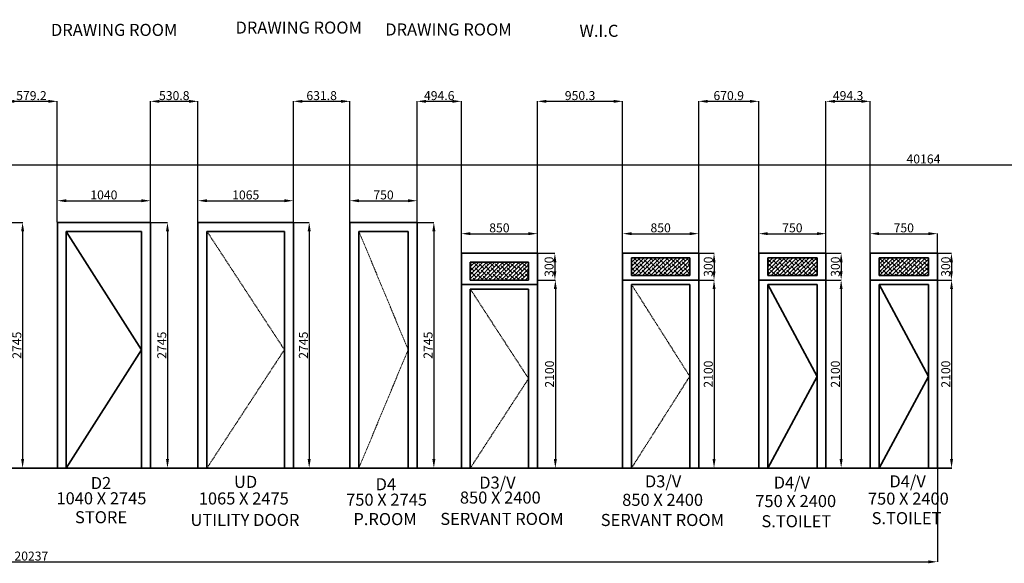
# Model space of a CAD drawing. Units: millimetres. Extents: x -850 to 42148, y -7352 to 4589.
# Tile 2 of 4: x 11314 to 22310, y -7352 to -1278. Entities that reach past the tile are written whole.
import ezdxf

# ---------------------------------------------------------------- set-up
doc = ezdxf.new("R2010")
doc.units = ezdxf.units.MM
doc.linetypes.add('DASHED', pattern=[19.05, 12.7, -6.35])
for name, color, linetype, lineweight in [('A-ANNO-DIMS', 2, 'Continuous', 18), ('A-ANNO-TEXT', 7, 'Continuous', 18), ('A-DOOR', 3, 'Continuous', 35), ('A-DOOR-OPNG', 3, 'DASHED', 18), ('A-DOOR-PATT', 252, 'Continuous', 13)]:
    doc.layers.add(name, color=color, linetype=linetype, lineweight=lineweight)
doc.styles.get("Standard").update_dxf_attribs({"font": 'arial.ttf'})
doc.dimstyles.new('ISO-25', dxfattribs={"dimtxt": 100, "dimasz": 100, "dimexe": 1.25, "dimexo": 0.625, "dimtad": 1, "dimtxsty": 'Standard', "dimcen": 2.5, "dimadec": 0, "dimazin": 0, "dimtfac": 1, "dimtmove": 0, "dimatfit": 3, "dimfxl": 1, "dimarcsym": 0})

# ---------------------------------------------------------------- blocks, each defined once
blk = doc.blocks.new('*D38')
at = {"layer": 'A-ANNO-DIMS', "color": 0, "lineweight": -2, "transparency": 16777216}
for p, q in [((11156, -3543), (11347, -3543)), ((11346, -3643), (11346, -6188)), ((11156, -6288), (11347, -6288))]:
    blk.add_line(p, q, dxfattribs=at)
at = {"layer": 'A-ANNO-DIMS', "color": 0, "lineweight": 30, "transparency": 16777216}
for points in [[(11330, -3643), (11363, -3643), (11346, -3543)], [(11330, -6188), (11363, -6188), (11346, -6288)]]:
    blk.add_solid(points, dxfattribs=at)
at = {"layer": 'Defpoints', "color": 0, "lineweight": 30, "transparency": 16777216}
for p in [(11155, -3543), (11155, -6288), (11346, -6288)]:
    blk.add_point(p, dxfattribs=at)
at = {"layer": 'A-ANNO-DIMS', "color": 0, "transparency": 16777216, "insert": (11295, -4915), "char_height": 100, "attachment_point": 5, "rotation": 90}
blk.add_mtext('2745', dxfattribs=at)
blk = doc.blocks.new('*D39')
at = {"layer": 'A-ANNO-DIMS', "color": 0, "lineweight": -2, "transparency": 16777216}
for p, q in [((11734, -3542), (11734, -3299)), ((11834, -3301), (12674, -3301)), ((12774, -3542), (12774, -3299))]:
    blk.add_line(p, q, dxfattribs=at)
at = {"layer": 'A-ANNO-DIMS', "color": 0, "lineweight": 30, "transparency": 16777216}
for points in [[(11834, -3284), (11834, -3317), (11734, -3301)], [(12674, -3284), (12674, -3317), (12774, -3301)]]:
    blk.add_solid(points, dxfattribs=at)
at = {"layer": 'Defpoints', "color": 0, "lineweight": 30, "transparency": 16777216}
for p in [(12774, -3301), (11734, -3543), (12774, -3543)]:
    blk.add_point(p, dxfattribs=at)
at = {"layer": 'A-ANNO-DIMS', "color": 0, "transparency": 16777216, "insert": (12254, -3249), "char_height": 100, "attachment_point": 5}
blk.add_mtext('1040', dxfattribs=at)
blk = doc.blocks.new('*D40')
at = {"layer": 'A-ANNO-DIMS', "color": 0, "lineweight": -2, "transparency": 16777216}
for p, q in [((12775, -3543), (12966, -3543)), ((12964, -3643), (12964, -6188)), ((12775, -6288), (12966, -6288))]:
    blk.add_line(p, q, dxfattribs=at)
at = {"layer": 'A-ANNO-DIMS', "color": 0, "lineweight": 30, "transparency": 16777216}
for points in [[(12948, -3643), (12981, -3643), (12964, -3543)], [(12948, -6188), (12981, -6188), (12964, -6288)]]:
    blk.add_solid(points, dxfattribs=at)
at = {"layer": 'Defpoints', "color": 0, "lineweight": 30, "transparency": 16777216}
for p in [(12774, -3543), (12774, -6288), (12964, -6288)]:
    blk.add_point(p, dxfattribs=at)
at = {"layer": 'A-ANNO-DIMS', "color": 0, "transparency": 16777216, "insert": (12913, -4915), "char_height": 100, "attachment_point": 5, "rotation": 90}
blk.add_mtext('2745', dxfattribs=at)
blk = doc.blocks.new('*D41')
at = {"layer": 'A-ANNO-DIMS', "color": 0, "lineweight": -2, "transparency": 16777216}
for p, q in [((13305, -3542), (13305, -3299)), ((13405, -3301), (14270, -3301)), ((14370, -3542), (14370, -3299))]:
    blk.add_line(p, q, dxfattribs=at)
at = {"layer": 'A-ANNO-DIMS', "color": 0, "lineweight": 30, "transparency": 16777216}
for points in [[(13405, -3284), (13405, -3317), (13305, -3301)], [(14270, -3284), (14270, -3317), (14370, -3301)]]:
    blk.add_solid(points, dxfattribs=at)
at = {"layer": 'Defpoints', "color": 0, "lineweight": 30, "transparency": 16777216}
for p in [(14370, -3301), (13305, -3543), (14370, -3543)]:
    blk.add_point(p, dxfattribs=at)
at = {"layer": 'A-ANNO-DIMS', "color": 0, "transparency": 16777216, "insert": (13838, -3249), "char_height": 100, "attachment_point": 5}
blk.add_mtext('1065', dxfattribs=at)
blk = doc.blocks.new('*D42')
at = {"layer": 'A-ANNO-DIMS', "color": 0, "lineweight": -2, "transparency": 16777216}
for p, q in [((14371, -3543), (14548, -3543)), ((14547, -3643), (14547, -6188)), ((14371, -6288), (14548, -6288))]:
    blk.add_line(p, q, dxfattribs=at)
at = {"layer": 'A-ANNO-DIMS', "color": 0, "lineweight": 30, "transparency": 16777216}
for points in [[(14530, -3643), (14564, -3643), (14547, -3543)], [(14530, -6188), (14564, -6188), (14547, -6288)]]:
    blk.add_solid(points, dxfattribs=at)
at = {"layer": 'Defpoints', "color": 0, "lineweight": 30, "transparency": 16777216}
for p in [(14370, -3543), (14370, -6288), (14547, -6288)]:
    blk.add_point(p, dxfattribs=at)
at = {"layer": 'A-ANNO-DIMS', "color": 0, "transparency": 16777216, "insert": (14495, -4915), "char_height": 100, "attachment_point": 5, "rotation": 90}
blk.add_mtext('2745', dxfattribs=at)
blk = doc.blocks.new('*D43')
at = {"layer": 'A-ANNO-DIMS', "color": 0, "lineweight": -2, "transparency": 16777216}
for p, q in [((15002, -3542), (15002, -3299)), ((15102, -3301), (15652, -3301)), ((15752, -3542), (15752, -3299))]:
    blk.add_line(p, q, dxfattribs=at)
at = {"layer": 'A-ANNO-DIMS', "color": 0, "lineweight": 30, "transparency": 16777216}
for points in [[(15102, -3284), (15102, -3317), (15002, -3301)], [(15652, -3284), (15652, -3317), (15752, -3301)]]:
    blk.add_solid(points, dxfattribs=at)
at = {"layer": 'Defpoints', "color": 0, "lineweight": 30, "transparency": 16777216}
for p in [(15752, -3301), (15002, -3543), (15752, -3543)]:
    blk.add_point(p, dxfattribs=at)
at = {"layer": 'A-ANNO-DIMS', "color": 0, "transparency": 16777216, "insert": (15377, -3249), "char_height": 100, "attachment_point": 5}
blk.add_mtext('750', dxfattribs=at)
blk = doc.blocks.new('*D44')
at = {"layer": 'A-ANNO-DIMS', "color": 0, "lineweight": -2, "transparency": 16777216}
for p, q in [((15752, -3543), (15940, -3543)), ((15939, -3643), (15939, -6188)), ((15752, -6288), (15940, -6288))]:
    blk.add_line(p, q, dxfattribs=at)
at = {"layer": 'A-ANNO-DIMS', "color": 0, "lineweight": 30, "transparency": 16777216}
for points in [[(15922, -3643), (15956, -3643), (15939, -3543)], [(15922, -6188), (15956, -6188), (15939, -6288)]]:
    blk.add_solid(points, dxfattribs=at)
at = {"layer": 'Defpoints', "color": 0, "lineweight": 30, "transparency": 16777216}
for p in [(15752, -3543), (15752, -6288), (15939, -6288)]:
    blk.add_point(p, dxfattribs=at)
at = {"layer": 'A-ANNO-DIMS', "color": 0, "transparency": 16777216, "insert": (15887, -4915), "char_height": 100, "attachment_point": 5, "rotation": 90}
blk.add_mtext('2745', dxfattribs=at)
blk = doc.blocks.new('*D45')
at = {"layer": 'A-ANNO-DIMS', "color": 0, "lineweight": -2, "transparency": 16777216}
for p, q in [((16246, -3887), (16246, -3667)), ((16346, -3669), (16996, -3669)), ((17096, -3887), (17096, -3667))]:
    blk.add_line(p, q, dxfattribs=at)
at = {"layer": 'A-ANNO-DIMS', "color": 0, "lineweight": 30, "transparency": 16777216}
for points in [[(16346, -3652), (16346, -3685), (16246, -3669)], [(16996, -3652), (16996, -3685), (17096, -3669)]]:
    blk.add_solid(points, dxfattribs=at)
at = {"layer": 'Defpoints', "color": 0, "lineweight": 30, "transparency": 16777216}
for p in [(17096, -3669), (16246, -3888), (17096, -3888)]:
    blk.add_point(p, dxfattribs=at)
at = {"layer": 'A-ANNO-DIMS', "color": 0, "transparency": 16777216, "insert": (16671, -3617), "char_height": 100, "attachment_point": 5}
blk.add_mtext('850', dxfattribs=at)
blk = doc.blocks.new('*D46')
at = {"layer": 'A-ANNO-DIMS', "color": 0, "lineweight": -2, "transparency": 16777216}
for p, q in [((17097, -4188), (17297, -4188)), ((17296, -4288), (17296, -6188)), ((17097, -6288), (17297, -6288))]:
    blk.add_line(p, q, dxfattribs=at)
at = {"layer": 'A-ANNO-DIMS', "color": 0, "lineweight": 30, "transparency": 16777216}
for points in [[(17279, -4288), (17313, -4288), (17296, -4188)], [(17279, -6188), (17313, -6188), (17296, -6288)]]:
    blk.add_solid(points, dxfattribs=at)
at = {"layer": 'Defpoints', "color": 0, "lineweight": 30, "transparency": 16777216}
for p in [(17096, -4188), (17096, -6288), (17296, -6288)]:
    blk.add_point(p, dxfattribs=at)
at = {"layer": 'A-ANNO-DIMS', "color": 0, "transparency": 16777216, "insert": (17244, -5238), "char_height": 100, "attachment_point": 5, "rotation": 90}
blk.add_mtext('2100', dxfattribs=at)
blk = doc.blocks.new('*D47')
at = {"layer": 'A-ANNO-DIMS', "color": 0, "lineweight": -2, "transparency": 16777216}
for p, q in [((17097, -3888), (17292, -3888)), ((17291, -3988), (17291, -4088)), ((17097, -4188), (17292, -4188))]:
    blk.add_line(p, q, dxfattribs=at)
at = {"layer": 'A-ANNO-DIMS', "color": 0, "lineweight": 30, "transparency": 16777216}
for points in [[(17274, -3988), (17307, -3988), (17291, -3888)], [(17274, -4088), (17307, -4088), (17291, -4188)]]:
    blk.add_solid(points, dxfattribs=at)
at = {"layer": 'Defpoints', "color": 0, "lineweight": 30, "transparency": 16777216}
for p in [(17096, -3888), (17096, -4188), (17291, -4188)]:
    blk.add_point(p, dxfattribs=at)
at = {"layer": 'A-ANNO-DIMS', "color": 0, "transparency": 16777216, "insert": (17239, -4038), "char_height": 100, "attachment_point": 5, "rotation": 90}
blk.add_mtext('300', dxfattribs=at)
blk = doc.blocks.new('*D48')
at = {"layer": 'A-ANNO-DIMS', "color": 0, "lineweight": -2, "transparency": 16777216}
for p, q in [((18047, -3887), (18047, -3667)), ((18147, -3669), (18797, -3669)), ((18897, -3887), (18897, -3667))]:
    blk.add_line(p, q, dxfattribs=at)
at = {"layer": 'A-ANNO-DIMS', "color": 0, "lineweight": 30, "transparency": 16777216}
for points in [[(18147, -3652), (18147, -3685), (18047, -3669)], [(18797, -3652), (18797, -3685), (18897, -3669)]]:
    blk.add_solid(points, dxfattribs=at)
at = {"layer": 'Defpoints', "color": 0, "lineweight": 30, "transparency": 16777216}
for p in [(18897, -3669), (18047, -3888), (18897, -3888)]:
    blk.add_point(p, dxfattribs=at)
at = {"layer": 'A-ANNO-DIMS', "color": 0, "transparency": 16777216, "insert": (18472, -3617), "char_height": 100, "attachment_point": 5}
blk.add_mtext('850', dxfattribs=at)
blk = doc.blocks.new('*D49')
at = {"layer": 'A-ANNO-DIMS', "color": 0, "lineweight": -2, "transparency": 16777216}
for p, q in [((18897, -3888), (19070, -3888)), ((19068, -3988), (19068, -4088)), ((18897, -4188), (19070, -4188))]:
    blk.add_line(p, q, dxfattribs=at)
at = {"layer": 'A-ANNO-DIMS', "color": 0, "lineweight": 30, "transparency": 16777216}
for points in [[(19052, -3988), (19085, -3988), (19068, -3888)], [(19052, -4088), (19085, -4088), (19068, -4188)]]:
    blk.add_solid(points, dxfattribs=at)
at = {"layer": 'Defpoints', "color": 0, "lineweight": 30, "transparency": 16777216}
for p in [(18897, -3888), (18897, -4188), (19068, -4188)]:
    blk.add_point(p, dxfattribs=at)
at = {"layer": 'A-ANNO-DIMS', "color": 0, "transparency": 16777216, "insert": (19017, -4038), "char_height": 100, "attachment_point": 5, "rotation": 90}
blk.add_mtext('300', dxfattribs=at)
blk = doc.blocks.new('*D50')
at = {"layer": 'A-ANNO-DIMS', "color": 0, "lineweight": -2, "transparency": 16777216}
for p, q in [((18897, -4188), (19070, -4188)), ((19068, -4288), (19068, -6188)), ((18897, -6288), (19070, -6288))]:
    blk.add_line(p, q, dxfattribs=at)
at = {"layer": 'A-ANNO-DIMS', "color": 0, "lineweight": 30, "transparency": 16777216}
for points in [[(19052, -4288), (19085, -4288), (19068, -4188)], [(19052, -6188), (19085, -6188), (19068, -6288)]]:
    blk.add_solid(points, dxfattribs=at)
at = {"layer": 'Defpoints', "color": 0, "lineweight": 30, "transparency": 16777216}
for p in [(18897, -4188), (18897, -6288), (19068, -6288)]:
    blk.add_point(p, dxfattribs=at)
at = {"layer": 'A-ANNO-DIMS', "color": 0, "transparency": 16777216, "insert": (19017, -5238), "char_height": 100, "attachment_point": 5, "rotation": 90}
blk.add_mtext('2100', dxfattribs=at)
blk = doc.blocks.new('*D51')
at = {"layer": 'A-ANNO-DIMS', "color": 0, "lineweight": -2, "transparency": 16777216}
for p, q in [((19568, -3887), (19568, -3667)), ((19668, -3669), (20218, -3669)), ((20318, -3887), (20318, -3667))]:
    blk.add_line(p, q, dxfattribs=at)
at = {"layer": 'A-ANNO-DIMS', "color": 0, "lineweight": 30, "transparency": 16777216}
for points in [[(19668, -3652), (19668, -3685), (19568, -3669)], [(20218, -3652), (20218, -3685), (20318, -3669)]]:
    blk.add_solid(points, dxfattribs=at)
at = {"layer": 'Defpoints', "color": 0, "lineweight": 30, "transparency": 16777216}
for p in [(20318, -3669), (19568, -3888), (20318, -3888)]:
    blk.add_point(p, dxfattribs=at)
at = {"layer": 'A-ANNO-DIMS', "color": 0, "transparency": 16777216, "insert": (19943, -3617), "char_height": 100, "attachment_point": 5}
blk.add_mtext('750', dxfattribs=at)
blk = doc.blocks.new('*D52')
at = {"layer": 'A-ANNO-DIMS', "color": 0, "lineweight": -2, "transparency": 16777216}
for p, q in [((20318, -3888), (20489, -3888)), ((20488, -3988), (20488, -4088)), ((20318, -4188), (20489, -4188))]:
    blk.add_line(p, q, dxfattribs=at)
at = {"layer": 'A-ANNO-DIMS', "color": 0, "lineweight": 30, "transparency": 16777216}
for points in [[(20471, -3988), (20504, -3988), (20488, -3888)], [(20471, -4088), (20504, -4088), (20488, -4188)]]:
    blk.add_solid(points, dxfattribs=at)
at = {"layer": 'Defpoints', "color": 0, "lineweight": 30, "transparency": 16777216}
for p in [(20318, -3888), (20318, -4188), (20488, -4188)]:
    blk.add_point(p, dxfattribs=at)
at = {"layer": 'A-ANNO-DIMS', "color": 0, "transparency": 16777216, "insert": (20436, -4038), "char_height": 100, "attachment_point": 5, "rotation": 90}
blk.add_mtext('300', dxfattribs=at)
blk = doc.blocks.new('*D53')
at = {"layer": 'A-ANNO-DIMS', "color": 0, "lineweight": -2, "transparency": 16777216}
for p, q in [((20318, -4188), (20489, -4188)), ((20488, -4288), (20488, -6188)), ((20318, -6288), (20489, -6288))]:
    blk.add_line(p, q, dxfattribs=at)
at = {"layer": 'A-ANNO-DIMS', "color": 0, "lineweight": 30, "transparency": 16777216}
for points in [[(20471, -4288), (20504, -4288), (20488, -4188)], [(20471, -6188), (20504, -6188), (20488, -6288)]]:
    blk.add_solid(points, dxfattribs=at)
at = {"layer": 'Defpoints', "color": 0, "lineweight": 30, "transparency": 16777216}
for p in [(20318, -4188), (20318, -6288), (20488, -6288)]:
    blk.add_point(p, dxfattribs=at)
at = {"layer": 'A-ANNO-DIMS', "color": 0, "transparency": 16777216, "insert": (20436, -5238), "char_height": 100, "attachment_point": 5, "rotation": 90}
blk.add_mtext('2100', dxfattribs=at)
blk = doc.blocks.new('*D54')
at = {"layer": 'A-ANNO-DIMS', "color": 0, "lineweight": -2, "transparency": 16777216}
for p, q in [((20812, -3887), (20812, -3667)), ((20912, -3669), (21462, -3669)), ((21562, -3887), (21562, -3667))]:
    blk.add_line(p, q, dxfattribs=at)
at = {"layer": 'A-ANNO-DIMS', "color": 0, "lineweight": 30, "transparency": 16777216}
for points in [[(20912, -3652), (20912, -3685), (20812, -3669)], [(21462, -3652), (21462, -3685), (21562, -3669)]]:
    blk.add_solid(points, dxfattribs=at)
at = {"layer": 'Defpoints', "color": 0, "lineweight": 30, "transparency": 16777216}
for p in [(21562, -3669), (20812, -3888), (21562, -3888)]:
    blk.add_point(p, dxfattribs=at)
at = {"layer": 'A-ANNO-DIMS', "color": 0, "transparency": 16777216, "insert": (21187, -3617), "char_height": 100, "attachment_point": 5}
blk.add_mtext('750', dxfattribs=at)
blk = doc.blocks.new('*D55')
at = {"layer": 'A-ANNO-DIMS', "color": 0, "lineweight": -2, "transparency": 16777216}
for p, q in [((21563, -3888), (21721, -3888)), ((21719, -3988), (21719, -4088)), ((21563, -4188), (21721, -4188))]:
    blk.add_line(p, q, dxfattribs=at)
at = {"layer": 'A-ANNO-DIMS', "color": 0, "lineweight": 30, "transparency": 16777216}
for points in [[(21703, -3988), (21736, -3988), (21719, -3888)], [(21703, -4088), (21736, -4088), (21719, -4188)]]:
    blk.add_solid(points, dxfattribs=at)
at = {"layer": 'Defpoints', "color": 0, "lineweight": 30, "transparency": 16777216}
for p in [(21562, -3888), (21562, -4188), (21719, -4188)]:
    blk.add_point(p, dxfattribs=at)
at = {"layer": 'A-ANNO-DIMS', "color": 0, "transparency": 16777216, "insert": (21668, -4038), "char_height": 100, "attachment_point": 5, "rotation": 90}
blk.add_mtext('300', dxfattribs=at)
blk = doc.blocks.new('*D56')
at = {"layer": 'A-ANNO-DIMS', "color": 0, "lineweight": -2, "transparency": 16777216}
for p, q in [((21563, -4188), (21722, -4188)), ((21721, -4288), (21721, -6188)), ((21563, -6288), (21722, -6288))]:
    blk.add_line(p, q, dxfattribs=at)
at = {"layer": 'A-ANNO-DIMS', "color": 0, "lineweight": 30, "transparency": 16777216}
for points in [[(21704, -4288), (21737, -4288), (21721, -4188)], [(21704, -6188), (21737, -6188), (21721, -6288)]]:
    blk.add_solid(points, dxfattribs=at)
at = {"layer": 'Defpoints', "color": 0, "lineweight": 30, "transparency": 16777216}
for p in [(21562, -4188), (21562, -6288), (21721, -6288)]:
    blk.add_point(p, dxfattribs=at)
at = {"layer": 'A-ANNO-DIMS', "color": 0, "transparency": 16777216, "insert": (21669, -5238), "char_height": 100, "attachment_point": 5, "rotation": 90}
blk.add_mtext('2100', dxfattribs=at)
blk = doc.blocks.new('DOOR-D2-1040')
for p, q in [((8473, -6288), (8473, -3543)), ((8473, -3543), (9513, -3543)), ((9513, -3543), (9513, -6288)), ((8573, -6288), (8573, -3643)), ((8573, -3643), (9413, -3643)), ((8573, -3643), (9413, -4965)), ((9413, -3643), (9413, -6288)), ((9413, -4965), (8573, -6288))]:
    blk.add_line(p, q)
blk = doc.blocks.new('DOOR-D4V-750')
for p, q in [((19568, -4188), (19568, -3888)), ((19568, -3888), (20318, -3888)), ((19668, -3938), (20218, -3938)), ((19668, -4138), (19668, -3938)), ((20218, -3938), (20218, -4138)), ((20318, -3888), (20318, -4188)), ((19668, -4138), (20218, -4138)), ((19568, -6288), (19568, -4188)), ((19568, -4188), (20318, -4188)), ((19668, -6288), (19668, -4238)), ((19668, -4238), (20218, -4238)), ((19668, -4238), (20218, -5263)), ((20218, -4238), (20218, -6288)), ((20318, -4188), (20318, -6288)), ((20218, -5263), (19668, -6288))]:
    blk.add_line(p, q)
blk = doc.blocks.new('*D60')
at = {"layer": 'A-ANNO-DIMS', "color": 0, "lineweight": -2, "transparency": 16777216}
for p, q in [((41489, -432), (41489, -2900)), ((1325, -812), (1325, -2900)), ((1425, -2899), (41389, -2899))]:
    blk.add_line(p, q, dxfattribs=at)
at = {"layer": 'A-ANNO-DIMS', "color": 0, "lineweight": 30, "transparency": 16777216}
for points in [[(1425, -2882), (1425, -2915), (1325, -2899)], [(41389, -2882), (41389, -2915), (41489, -2899)]]:
    blk.add_solid(points, dxfattribs=at)
at = {"layer": 'Defpoints', "color": 0, "lineweight": 30, "transparency": 16777216}
for p in [(41489, -431), (1325, -811), (41489, -2899)]:
    blk.add_point(p, dxfattribs=at)
at = {"layer": 'A-ANNO-DIMS', "color": 0, "transparency": 16777216, "insert": (21407, -2847), "char_height": 100, "attachment_point": 5}
blk.add_mtext('40164', dxfattribs=at)
blk = doc.blocks.new('*D83')
at = {"layer": 'A-ANNO-DIMS', "color": 0, "lineweight": -2, "transparency": 16777216}
for p, q in [((1325, -3238), (1325, -7337)), ((21562, -6288), (21562, -7337)), ((1425, -7335), (21462, -7335))]:
    blk.add_line(p, q, dxfattribs=at)
at = {"layer": 'A-ANNO-DIMS', "color": 0, "lineweight": 30, "transparency": 16777216}
for points in [[(1425, -7319), (1425, -7352), (1325, -7335)], [(21462, -7319), (21462, -7352), (21562, -7335)]]:
    blk.add_solid(points, dxfattribs=at)
at = {"layer": 'Defpoints', "color": 0, "lineweight": 30, "transparency": 16777216}
for p in [(1325, -3238), (21562, -6288), (21562, -7335)]:
    blk.add_point(p, dxfattribs=at)
at = {"layer": 'A-ANNO-DIMS', "color": 0, "transparency": 16777216, "insert": (11444, -7284), "char_height": 100, "attachment_point": 5}
blk.add_mtext('20237', dxfattribs=at)
blk = doc.blocks.new('*D88')
at = {"layer": 'A-ANNO-DIMS', "color": 0, "lineweight": -2, "transparency": 16777216}
for p, q in [((11155, -3542), (11155, -2189)), ((11255, -2190), (11634, -2190)), ((11734, -3542), (11734, -2189))]:
    blk.add_line(p, q, dxfattribs=at)
at = {"layer": 'A-ANNO-DIMS', "color": 0, "lineweight": 30, "transparency": 16777216}
for points in [[(11255, -2174), (11255, -2207), (11155, -2190)], [(11634, -2174), (11634, -2207), (11734, -2190)]]:
    blk.add_solid(points, dxfattribs=at)
at = {"layer": 'Defpoints', "color": 0, "lineweight": 30, "transparency": 16777216}
for p in [(11734, -2190), (11155, -3543), (11734, -3543)]:
    blk.add_point(p, dxfattribs=at)
at = {"layer": 'A-ANNO-DIMS', "color": 0, "transparency": 16777216, "insert": (11445, -2139), "char_height": 100, "attachment_point": 5}
blk.add_mtext('579.2', dxfattribs=at)
blk = doc.blocks.new('*D89')
at = {"layer": 'A-ANNO-DIMS', "color": 0, "lineweight": -2, "transparency": 16777216}
for p, q in [((12774, -3542), (12774, -2189)), ((12874, -2190), (13205, -2190)), ((13305, -3542), (13305, -2189))]:
    blk.add_line(p, q, dxfattribs=at)
at = {"layer": 'A-ANNO-DIMS', "color": 0, "lineweight": 30, "transparency": 16777216}
for points in [[(12874, -2174), (12874, -2207), (12774, -2190)], [(13205, -2174), (13205, -2207), (13305, -2190)]]:
    blk.add_solid(points, dxfattribs=at)
at = {"layer": 'Defpoints', "color": 0, "lineweight": 30, "transparency": 16777216}
for p in [(13305, -2190), (12774, -3543), (13305, -3543)]:
    blk.add_point(p, dxfattribs=at)
at = {"layer": 'A-ANNO-DIMS', "color": 0, "transparency": 16777216, "insert": (13040, -2139), "char_height": 100, "attachment_point": 5}
blk.add_mtext('530.8', dxfattribs=at)
blk = doc.blocks.new('*D90')
at = {"layer": 'A-ANNO-DIMS', "color": 0, "lineweight": -2, "transparency": 16777216}
for p, q in [((14370, -3542), (14370, -2189)), ((14470, -2190), (14902, -2190)), ((15002, -3542), (15002, -2189))]:
    blk.add_line(p, q, dxfattribs=at)
at = {"layer": 'A-ANNO-DIMS', "color": 0, "lineweight": 30, "transparency": 16777216}
for points in [[(14470, -2174), (14470, -2207), (14370, -2190)], [(14902, -2174), (14902, -2207), (15002, -2190)]]:
    blk.add_solid(points, dxfattribs=at)
at = {"layer": 'Defpoints', "color": 0, "lineweight": 30, "transparency": 16777216}
for p in [(15002, -2190), (14370, -3543), (15002, -3543)]:
    blk.add_point(p, dxfattribs=at)
at = {"layer": 'A-ANNO-DIMS', "color": 0, "transparency": 16777216, "insert": (14686, -2139), "char_height": 100, "attachment_point": 5}
blk.add_mtext('631.8', dxfattribs=at)
blk = doc.blocks.new('*D91')
at = {"layer": 'A-ANNO-DIMS', "color": 0, "lineweight": -2, "transparency": 16777216}
for p, q in [((15752, -3542), (15752, -2189)), ((15852, -2190), (16146, -2190)), ((16246, -3887), (16246, -2189))]:
    blk.add_line(p, q, dxfattribs=at)
at = {"layer": 'A-ANNO-DIMS', "color": 0, "lineweight": 30, "transparency": 16777216}
for points in [[(15852, -2174), (15852, -2207), (15752, -2190)], [(16146, -2174), (16146, -2207), (16246, -2190)]]:
    blk.add_solid(points, dxfattribs=at)
at = {"layer": 'Defpoints', "color": 0, "lineweight": 30, "transparency": 16777216}
for p in [(16246, -2190), (15752, -3543), (16246, -3888)]:
    blk.add_point(p, dxfattribs=at)
at = {"layer": 'A-ANNO-DIMS', "color": 0, "transparency": 16777216, "insert": (15999, -2139), "char_height": 100, "attachment_point": 5}
blk.add_mtext('494.6', dxfattribs=at)
blk = doc.blocks.new('*D92')
at = {"layer": 'A-ANNO-DIMS', "color": 0, "lineweight": -2, "transparency": 16777216}
for p, q in [((17096, -3887), (17096, -2189)), ((17196, -2190), (17947, -2190)), ((18047, -3887), (18047, -2189))]:
    blk.add_line(p, q, dxfattribs=at)
at = {"layer": 'A-ANNO-DIMS', "color": 0, "lineweight": 30, "transparency": 16777216}
for points in [[(17196, -2174), (17196, -2207), (17096, -2190)], [(17947, -2174), (17947, -2207), (18047, -2190)]]:
    blk.add_solid(points, dxfattribs=at)
at = {"layer": 'Defpoints', "color": 0, "lineweight": 30, "transparency": 16777216}
for p in [(18047, -2190), (17096, -3888), (18047, -3888)]:
    blk.add_point(p, dxfattribs=at)
at = {"layer": 'A-ANNO-DIMS', "color": 0, "transparency": 16777216, "insert": (17572, -2139), "char_height": 100, "attachment_point": 5}
blk.add_mtext('950.3', dxfattribs=at)
blk = doc.blocks.new('*D93')
at = {"layer": 'A-ANNO-DIMS', "color": 0, "lineweight": -2, "transparency": 16777216}
for p, q in [((18897, -3887), (18897, -2189)), ((18997, -2190), (19468, -2190)), ((19568, -3887), (19568, -2189))]:
    blk.add_line(p, q, dxfattribs=at)
at = {"layer": 'A-ANNO-DIMS', "color": 0, "lineweight": 30, "transparency": 16777216}
for points in [[(18997, -2174), (18997, -2207), (18897, -2190)], [(19468, -2174), (19468, -2207), (19568, -2190)]]:
    blk.add_solid(points, dxfattribs=at)
at = {"layer": 'Defpoints', "color": 0, "lineweight": 30, "transparency": 16777216}
for p in [(19568, -2190), (18897, -3888), (19568, -3888)]:
    blk.add_point(p, dxfattribs=at)
at = {"layer": 'A-ANNO-DIMS', "color": 0, "transparency": 16777216, "insert": (19232, -2139), "char_height": 100, "attachment_point": 5}
blk.add_mtext('670.9', dxfattribs=at)
blk = doc.blocks.new('*D94')
at = {"layer": 'A-ANNO-DIMS', "color": 0, "lineweight": -2, "transparency": 16777216}
for p, q in [((20318, -3887), (20318, -2189)), ((20418, -2190), (20712, -2190)), ((20812, -3887), (20812, -2189))]:
    blk.add_line(p, q, dxfattribs=at)
at = {"layer": 'A-ANNO-DIMS', "color": 0, "lineweight": 30, "transparency": 16777216}
for points in [[(20418, -2174), (20418, -2207), (20318, -2190)], [(20712, -2174), (20712, -2207), (20812, -2190)]]:
    blk.add_solid(points, dxfattribs=at)
at = {"layer": 'Defpoints', "color": 0, "lineweight": 30, "transparency": 16777216}
for p in [(20812, -2190), (20318, -3888), (20812, -3888)]:
    blk.add_point(p, dxfattribs=at)
at = {"layer": 'A-ANNO-DIMS', "color": 0, "transparency": 16777216, "insert": (20565, -2139), "char_height": 100, "attachment_point": 5}
blk.add_mtext('494.3', dxfattribs=at)

msp = doc.modelspace()

# ---------------------------------------------------------------- hatches: boundary and pattern name
at = {"layer": 'A-DOOR-PATT'}
h = msp.add_hatch(dxfattribs=at)
h.set_pattern_fill('ANSI38', color=256, scale=10)
h.paths.add_polyline_path([(16996.454, -3987.868), (16346.454, -3987.868), (16346.454, -4187.868), (16996.454, -4187.868)])
h.paths.add_polyline_path([(18796.794, -3937.868), (18146.794, -3937.868), (18146.794, -4137.868), (18796.794, -4137.868)])
h.paths.add_polyline_path([(20217.652, -3937.868), (19667.652, -3937.868), (19667.652, -4137.868), (20217.652, -4137.868)])
h.paths.add_polyline_path([(21461.986, -3937.868), (20911.986, -3937.868), (20911.986, -4137.868), (21461.986, -4137.868)])

# ---------------------------------------------------------------- linework, layer by layer
at = {"layer": 'A-DOOR'}
for p, q in [((13305.029, -6287.868), (13305.029, -3542.868)), ((13305.029, -3542.868), (14370.029, -3542.868)), ((14370.029, -3542.868), (14370.029, -6287.868)), ((15001.845, -6287.868), (15001.845, -3542.868)), ((15001.845, -3542.868), (15751.845, -3542.868)), ((15751.845, -3542.868), (15751.845, -6287.868)), ((13405.029, -6287.868), (13405.029, -3642.868)), ((13405.029, -3642.868), (14270.029, -3642.868)), ((14270.029, -3642.868), (14270.029, -6287.868)), ((15101.845, -6287.868), (15101.845, -3642.868)), ((15101.845, -3642.868), (15651.845, -3642.868)), ((15651.845, -3642.868), (15651.845, -6287.868)), ((16246.454, -6287.868), (16246.454, -3887.868)), ((16246.454, -3887.868), (17096.454, -3887.868)), ((17096.454, -3887.868), (17096.454, -6287.868)), ((18046.794, -4187.868), (18046.794, -3887.868)), ((18046.794, -3887.868), (18896.794, -3887.868)), ((18146.794, -3937.868), (18796.794, -3937.868)), ((18146.794, -4137.868), (18146.794, -3937.868)), ((18796.794, -3937.868), (18796.794, -4137.868)), ((18896.794, -3887.868), (18896.794, -4187.868)), ((16346.454, -3987.868), (16996.454, -3987.868)), ((16346.454, -4187.868), (16346.454, -3987.868)), ((16996.454, -3987.868), (16996.454, -4187.868)), ((18146.794, -4137.868), (18796.794, -4137.868)), ((17096.454, -4237.868), (16246.454, -4237.868)), ((16246.454, -4237.868), (16246.454, -4237.868)), ((16346.454, -4187.868), (16996.454, -4187.868)), ((16346.454, -6287.868), (16346.454, -4287.868)), ((16346.454, -4287.868), (16996.454, -4287.868)), ((16996.454, -4287.868), (16996.454, -6287.868)), ((18046.794, -6287.868), (18046.794, -4187.868)), ((18046.794, -4187.868), (18896.794, -4187.868)), ((18146.794, -6287.868), (18146.794, -4237.868)), ((18146.794, -4237.868), (18796.794, -4237.868)), ((18796.794, -4237.868), (18796.794, -6287.868)), ((18896.794, -4187.868), (18896.794, -6287.868)), ((1325.061, -6287.868), (21721.958, -6287.868)), ((18046.794, -6287.868), (18046.794, -6285.868))]:
    msp.add_line(p, q, dxfattribs=at)
at = {"layer": 'A-DOOR-OPNG'}
for p, q in [((13405.029, -3642.868), (14270.029, -4965.368)), ((15101.845, -3642.868), (15651.845, -4965.368)), ((16346.454, -4287.868), (16996.454, -5287.868)), ((18146.794, -4237.868), (18796.794, -5262.868)), ((14270.029, -4965.368), (13405.029, -6287.868)), ((15651.845, -4965.368), (15101.845, -6287.868)), ((18796.794, -5262.868), (18146.794, -6287.868)), ((16996.454, -5287.868), (16346.454, -6287.868))]:
    msp.add_line(p, q, dxfattribs=at)

# ---------------------------------------------------------------- block references
at = {"layer": 'A-DOOR'}
for name, p in [('DOOR-D2-1040', (3261.345, 0)), ('DOOR-D4V-750', (0, 0)), ('DOOR-D4V-750', (1244.334, 0))]:
    msp.add_blockref(name, p, dxfattribs=at)

# ---------------------------------------------------------------- texts
at = {"layer": 'A-ANNO-TEXT'}
for s, height, p in [('DRAWING ROOM', 134.88886, (13724.128, -1433.696)), ('DRAWING ROOM', 134.88886, (15396.245, -1454.785)), ('DRAWING ROOM', 134.88886, (11662.879, -1459.312)), ('W.I.C', 134.8889, (17564.9, -1469.579)), ('UD', 134.8889, (13707.241, -6509.119)), ('D3/V', 134.8889, (16445.796, -6517.389)), ('D3/V', 134.8889, (18295.928, -6503.709)), ('D4/V', 134.8889, (19734.252, -6517.389)), ('D4/V', 134.8889, (21026.573, -6503.709)), ('D2', 134.8889, (12107.385, -6522.56)), ('D4', 134.8889, (15288.372, -6535.793)), ('1040 X 2745', 134.88886, (11724.374, -6692.976)), ('1065 X 2475', 134.88886, (13314.008, -6695.047)), ('750 X 2745', 134.8889, (14959.403, -6708.575)), ('850 X 2400', 134.8889, (16229.921, -6684.68)), ('850 X 2400', 134.8889, (18042.591, -6710.157)), ('750 X 2400', 134.8889, (19528.844, -6723.838)), ('750 X 2400', 134.8889, (20786.93, -6696.477)), ('STORE', 134.8889, (11931.407, -6904.423)), ('UTILITY DOOR', 134.88886, (13221.128, -6934.407)), ('P.ROOM', 134.8889, (15040.456, -6925.325)), ('SERVANT ROOM', 134.88886, (16010.991, -6923.282)), ('SERVANT ROOM', 134.88886, (17802.948, -6935.285)), ('S.TOILET', 134.8889, (19597.313, -6948.965)), ('S.TOILET', 134.8889, (20828.012, -6914.764))]:
    msp.add_text(s, height=height, dxfattribs=at).set_placement(p)

# ---------------------------------------------------------------- dimensions: what is measured, and where the dimension line sits
at = {"layer": 'A-ANNO-DIMS'}
for base, p1, p2, override, picture, middle in [((41488.766, -2898.624), (1325.061, -811.124), (41488.766, -431.124), {"dimdec": 0, "dimlfac": 1, "dimrnd": 0, "dimzin": 0, "dimdsep": 46, "dimlunit": 2}, '*D60', (21406.913, -2846.942)), ((11734.228, -2190.368), (11155.027, -3542.868), (11734.228, -3542.868), {"dimdec": 1, "dimlfac": 1, "dimrnd": 0, "dimzin": 0, "dimdsep": 46, "dimlunit": 2}, '*D88', (11444.627, -2138.685)), ((13305.029, -2190.368), (12774.228, -3542.868), (13305.029, -3542.868), {"dimdec": 1, "dimlfac": 1, "dimrnd": 0, "dimzin": 0, "dimdsep": 46, "dimlunit": 2}, '*D89', (13039.628, -2138.651)), ((15001.845, -2190.368), (14370.029, -3542.868), (15001.845, -3542.868), {"dimdec": 1, "dimlfac": 1, "dimrnd": 0, "dimzin": 0, "dimdsep": 46, "dimlunit": 2}, '*D90', (14685.937, -2138.651)), ((16246.454, -2190.368), (15751.845, -3542.868), (16246.454, -3887.868), {"dimdec": 1, "dimlfac": 1, "dimrnd": 0, "dimzin": 0, "dimdsep": 46, "dimlunit": 2}, '*D91', (15999.149, -2138.685)), ((18046.794, -2190.368), (17096.454, -3887.868), (18046.794, -3887.868), {"dimdec": 1, "dimlfac": 1, "dimrnd": 0, "dimzin": 0, "dimdsep": 46, "dimlunit": 2}, '*D92', (17571.624, -2138.651)), ((19567.652, -2190.368), (18896.794, -3887.868), (19567.652, -3887.868), {"dimdec": 1, "dimlfac": 1, "dimrnd": 0, "dimzin": 0, "dimdsep": 46, "dimlunit": 2}, '*D93', (19232.223, -2138.685)), ((20811.986, -2190.368), (20317.652, -3887.868), (20811.986, -3887.868), {"dimdec": 1, "dimlfac": 1, "dimrnd": 0, "dimzin": 0, "dimdsep": 46, "dimlunit": 2}, '*D94', (20564.819, -2138.651)), ((12774.228, -3300.609), (11734.228, -3542.868), (12774.228, -3542.868), {"dimclrd": 0, "dimclre": 0, "dimclrt": 0}, '*D39', (12254.228, -3248.927)), ((14370.029, -3300.609), (13305.029, -3542.868), (14370.029, -3542.868), {"dimclrd": 0, "dimclre": 0, "dimclrt": 0}, '*D41', (13837.529, -3248.927)), ((15751.845, -3300.609), (15001.845, -3542.868), (15751.845, -3542.868), {"dimclrd": 0, "dimclre": 0, "dimclrt": 0}, '*D43', (15376.845, -3248.927)), ((21561.986, -7335.368), (1325.061, -3237.868), (21561.986, -6287.868), {"dimdec": 0, "dimlfac": 1, "dimrnd": 0, "dimzin": 0, "dimdsep": 46, "dimlunit": 2}, '*D83', (11443.523, -7283.651)), ((17096.454, -3668.61), (16246.454, -3887.868), (17096.454, -3887.868), {"dimclrd": 0, "dimclre": 0, "dimclrt": 0}, '*D45', (16671.454, -3616.928)), ((18896.794, -3668.61), (18046.794, -3887.868), (18896.794, -3887.868), {"dimclrd": 0, "dimclre": 0, "dimclrt": 0}, '*D48', (18471.794, -3616.928)), ((20317.652, -3668.61), (19567.652, -3887.868), (20317.652, -3887.868), {"dimclrd": 0, "dimclre": 0, "dimclrt": 0}, '*D51', (19942.652, -3616.928)), ((21561.986, -3668.61), (20811.986, -3887.868), (21561.986, -3887.868), {"dimclrd": 0, "dimclre": 0, "dimclrt": 0}, '*D54', (21186.986, -3616.928))]:
    dim = msp.add_linear_dim(base=base, p1=p1, p2=p2, dimstyle='ISO-25', override=override, dxfattribs=at)
    dim.commit()
    dim.dimension.update_dxf_attribs({"geometry": picture, "text_midpoint": middle})
for base, p1, p2, picture, middle in [((11346.2, -6287.868), (11155.027, -3542.868), (11155.027, -6287.868), '*D38', (11294.518, -4915.368)), ((12964.273, -6287.868), (12774.228, -3542.868), (12774.228, -6287.868), '*D40', (12912.591, -4915.368)), ((14546.883, -6287.868), (14370.029, -3542.868), (14370.029, -6287.868), '*D42', (14495.201, -4915.368)), ((15938.871, -6287.868), (15751.845, -3542.868), (15751.845, -6287.868), '*D44', (15887.189, -4915.368)), ((17290.533, -4187.868), (17096.454, -3887.868), (17096.454, -4187.868), '*D47', (17238.817, -4037.868)), ((19068.452, -4187.868), (18896.794, -3887.868), (18896.794, -4187.868), '*D49', (19016.736, -4037.868)), ((20487.691, -4187.868), (20317.652, -3887.868), (20317.652, -4187.868), '*D52', (20435.975, -4037.868)), ((21719.458, -4187.868), (21561.986, -3887.868), (21561.986, -4187.868), '*D55', (21667.742, -4037.868)), ((17295.924, -6287.868), (17096.454, -4187.868), (17096.454, -6287.868), '*D46', (17244.242, -5237.868)), ((19068.452, -6287.868), (18896.794, -4187.868), (18896.794, -6287.868), '*D50', (19016.77, -5237.868)), ((20487.691, -6287.868), (20317.652, -4187.868), (20317.652, -6287.868), '*D53', (20436.009, -5237.868)), ((21720.708, -6287.868), (21561.986, -4187.868), (21561.986, -6287.868), '*D56', (21669.026, -5237.868))]:
    dim = msp.add_linear_dim(base=base, p1=p1, p2=p2, angle=90, dimstyle='ISO-25', override={"dimclrd": 0, "dimclre": 0, "dimclrt": 0}, dxfattribs=at)
    dim.commit()
    dim.dimension.update_dxf_attribs({"geometry": picture, "text_midpoint": middle})

doc.saveas('drawing.dxf')
